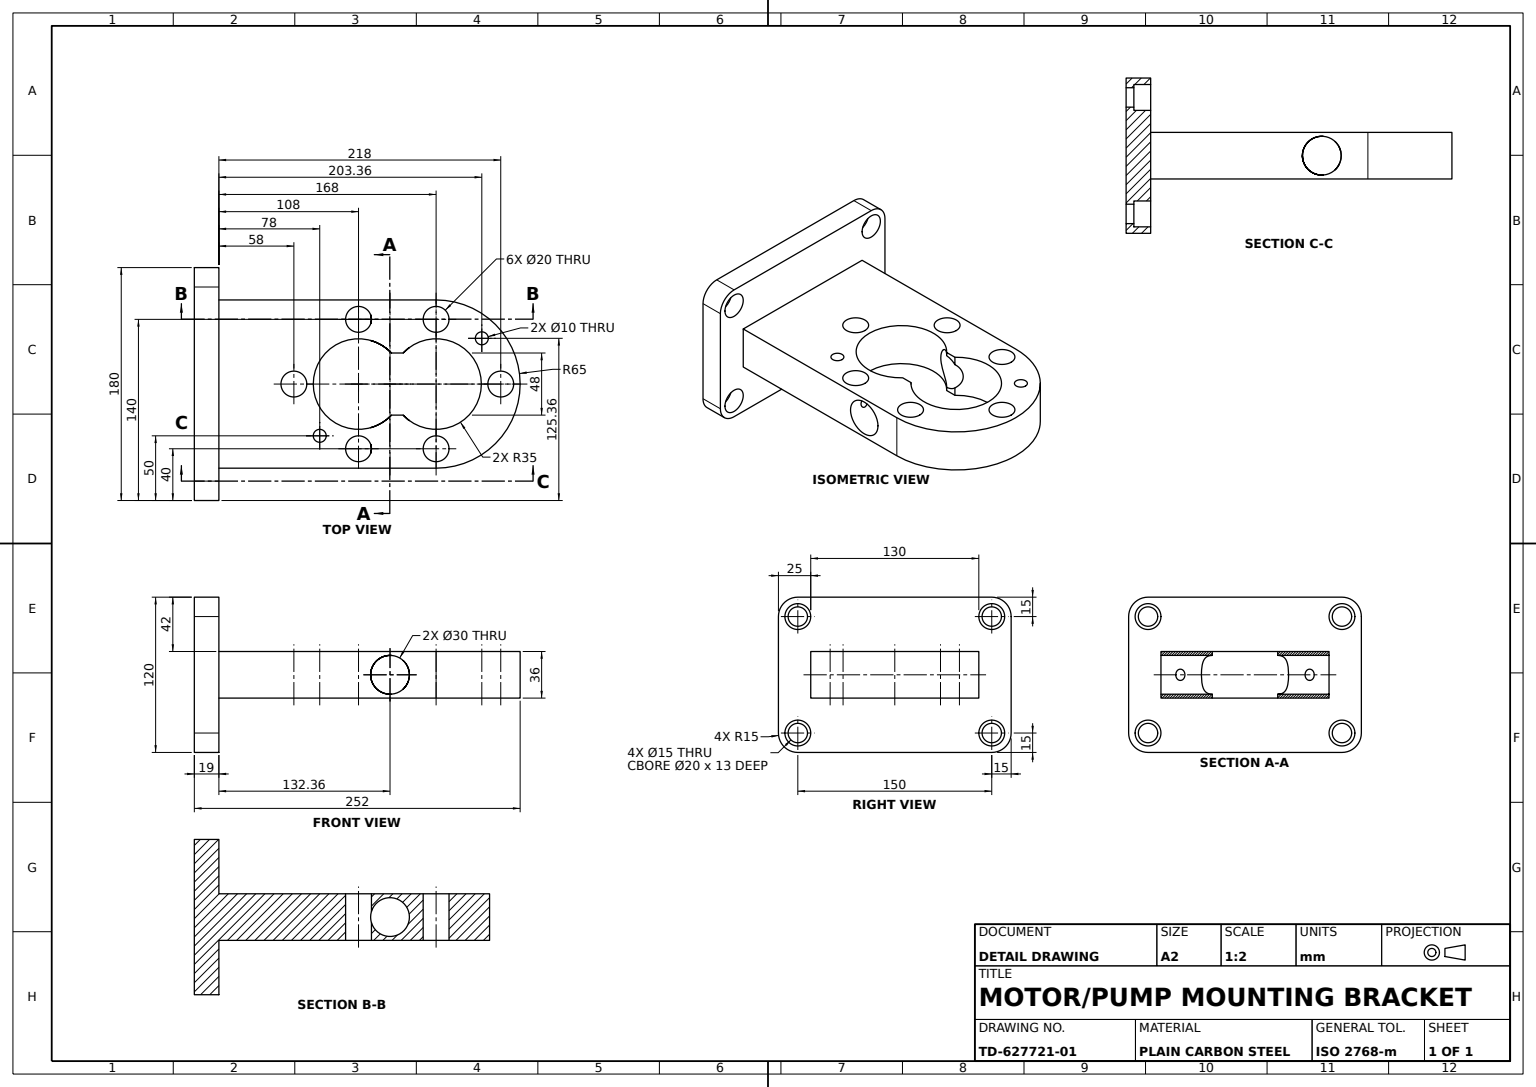
from build123d import *

# Parameters (mm, degrees)
FLANGE_PROFILE_SKETCH_W                = 180
FLANGE_PROFILE_SKETCH_H                = 120
MOUNTING_FLANGE_DEPTH                  = 19
SUPPORT_ARM_DEPTH                      = 18
BEARING_BORE_AND_BOLT_HOLES_SKETCH_R   = 10
BEARING_BORE_AND_BOLT_HOLES_SKETCH_R_2 = 5
BEARING_BORE_AND_BOLT_HOLES_DEPTH      = 36
CROSS_HOLE_SKETCH_R                    = 15
CROSS_HOLE_30_DEPTH                    = 305.489737101
FLANGE_CORNER_FILLETS_R15_R            = 15
FLANGE_MOUNTING_HOLES_SKETCH_R         = 7.5
FLANGE_MOUNTING_HOLES_DEPTH            = 36
FLANGE_SECONDARY_CUT_SKETCH_R          = 10
FLANGE_SECONDARY_CUT_DEPTH             = 13


with BuildPart() as part:
    # Flange Profile Sketch → Mounting Flange (new body)
    with BuildSketch(Plane.XY):
        with Locations((90, 60)):
            Rectangle(FLANGE_PROFILE_SKETCH_W, FLANGE_PROFILE_SKETCH_H)
    extrude(amount=MOUNTING_FLANGE_DEPTH)

    # Support Arm Profile Sketch → Support Arm (add, symmetric)
    with BuildSketch(Plane(origin=(0, 60, 0), x_dir=(1, 0, 0), z_dir=(0, 1, 0))):
        with BuildLine():
            Line((25, 168), (25, 0))
            Line((25, 0), (155, 0))
            Line((155, 0), (155, 168))
            ThreePointArc((155, 168), (90, 233), (25, 168))
        make_face()
    extrude(amount=SUPPORT_ARM_DEPTH, both=True)

    # Bearing Bore and Bolt Holes Sketch → Bearing Bore and Bolt Holes (cut)
    with BuildSketch(Plane(origin=(0, 78, 0), x_dir=(1, 0, 0), z_dir=(0, 1, 0))):
        with Locations(Location((90, 218, 0), (0, 0, 270))):
            Circle(BEARING_BORE_AND_BOLT_HOLES_SKETCH_R)
        with Locations(Location((140, 168, 0), (0, 0, 270))):
            Circle(BEARING_BORE_AND_BOLT_HOLES_SKETCH_R)
        with Locations(Location((40, 168, 0), (0, 0, 270))):
            Circle(BEARING_BORE_AND_BOLT_HOLES_SKETCH_R)
        with Locations(Location((90, 58, 0), (0, 0, 270))):
            Circle(BEARING_BORE_AND_BOLT_HOLES_SKETCH_R)
        with Locations(Location((40, 108, 0), (0, 0, 270))):
            Circle(BEARING_BORE_AND_BOLT_HOLES_SKETCH_R)
        with Locations(Location((140, 108, 0), (0, 0, 270))):
            Circle(BEARING_BORE_AND_BOLT_HOLES_SKETCH_R)
        with Locations(Location((54.644660941, 203.355339059, 0), (0, 0, 270))):
            Circle(BEARING_BORE_AND_BOLT_HOLES_SKETCH_R_2)
        with Locations(Location((130, 78, 0), (0, 0, 270))):
            Circle(BEARING_BORE_AND_BOLT_HOLES_SKETCH_R_2)
        with BuildLine():
            Line((66, 142.524521594), (66, 133.475478406))
            ThreePointArc((66, 133.475478406), (90, 73), (114, 133.475478406))
            Line((114, 133.475478406), (114, 142.524521594))
            ThreePointArc((114, 142.524521594), (90, 203), (66, 142.524521594))
        make_face()
    extrude(amount=-BEARING_BORE_AND_BOLT_HOLES_DEPTH, mode=Mode.SUBTRACT)

    # Cross Hole Sketch → Cross Hole Ø30 (cut, through all)
    with BuildSketch(Plane.ZY.offset(-25)):
        with Locations((-132.357693154, 60)):
            Circle(CROSS_HOLE_SKETCH_R)
    extrude(amount=-CROSS_HOLE_30_DEPTH, mode=Mode.SUBTRACT)

    # Flange Corner Fillets R15
    flange_corner_fillets_r15_edges = [part.edges().sort_by_distance(p)[0] for p in [
        (0, 120, 9.5),
        (180, 120, 9.5),
        (180, 0, 9.5),
        (0, 0, 9.5),
    ]]
    fillet(flange_corner_fillets_r15_edges, radius=FLANGE_CORNER_FILLETS_R15_R)

    # Flange Mounting Holes Sketch → Flange Mounting Holes (cut)
    with BuildSketch(Plane(origin=(0, 0, 0), x_dir=(-1, 0, 0), z_dir=(0, 0, -1))):
        with Locations((-165, 15)):
            Circle(FLANGE_MOUNTING_HOLES_SKETCH_R)
        with Locations((-15, 15)):
            Circle(FLANGE_MOUNTING_HOLES_SKETCH_R)
        with Locations((-15, 105)):
            Circle(FLANGE_MOUNTING_HOLES_SKETCH_R)
        with Locations((-165, 105)):
            Circle(FLANGE_MOUNTING_HOLES_SKETCH_R)
    extrude(amount=-FLANGE_MOUNTING_HOLES_DEPTH, mode=Mode.SUBTRACT)

    # Flange Secondary Cut Sketch → Flange Secondary Cut (cut)
    with BuildSketch(Plane(origin=(0, 0, 0), x_dir=(-1, 0, 0), z_dir=(0, 0, -1))):
        with Locations((-165, 105)):
            Circle(FLANGE_SECONDARY_CUT_SKETCH_R)
        with Locations((-15, 105)):
            Circle(FLANGE_SECONDARY_CUT_SKETCH_R)
        with Locations((-15, 15)):
            Circle(FLANGE_SECONDARY_CUT_SKETCH_R)
        with Locations((-165, 15)):
            Circle(FLANGE_SECONDARY_CUT_SKETCH_R)
    extrude(amount=-FLANGE_SECONDARY_CUT_DEPTH, mode=Mode.SUBTRACT)


solid = part.part
